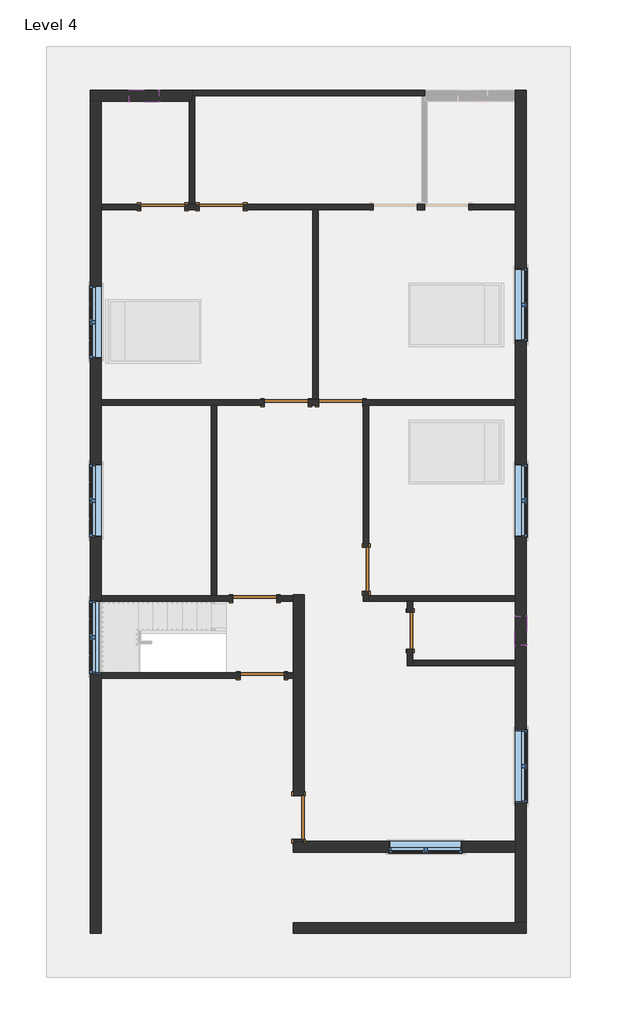
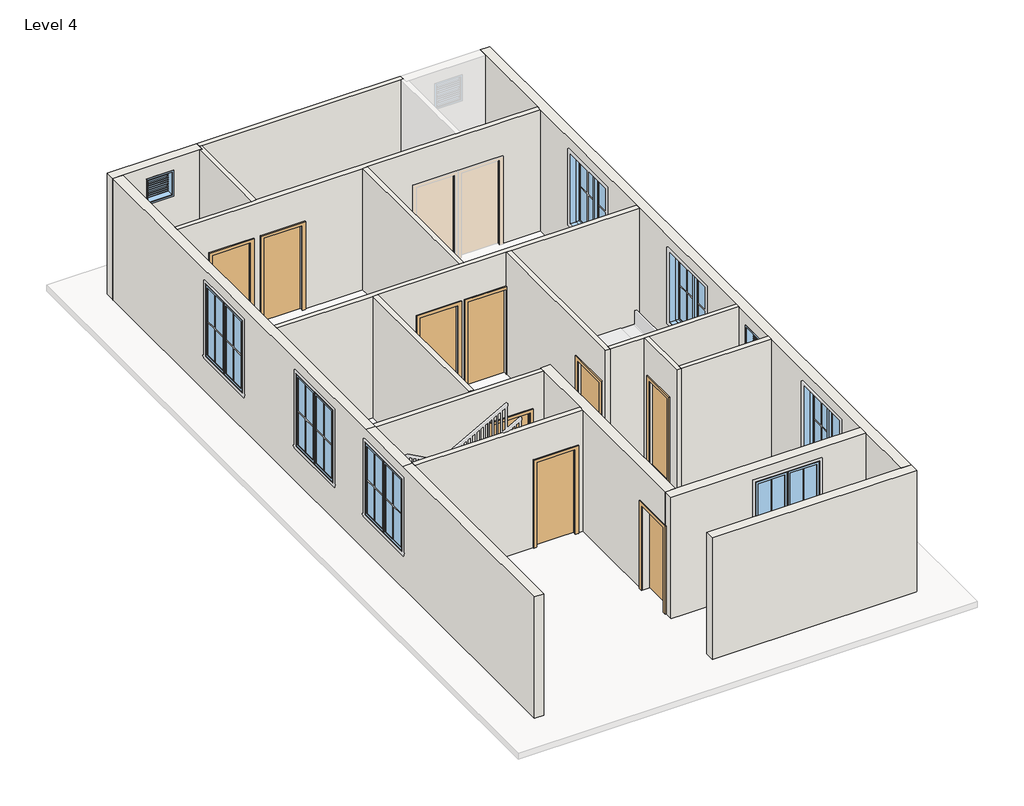
# One storey, part 1 of 3: 18 walls, 9 doors, 9 windows.
"""IFC4 building model written with IfcOpenShell, lengths in millimetres."""

from ifc_helpers import new_model, si_unit, frame, origin, place, context, project, spatial, polyline, outline, extrude, faceted_brep, transform, mapped, element, save
from components import door_78caadf7, single_flush_door_3_e5f9f3c4, single_flush_door_3_305aa2a5, single_flush_door_3_0ca8825f, window_casement_double_win_5_f93960c7, window_f2d8fef0

model = new_model("IFC4")

# Units and contexts
model_context = context("Model", 3, world=origin())
ifc_project = project(units=[si_unit("LENGTHUNIT", "METRE", prefix="MILLI")], contexts=[model_context])

# Site, building, storey
site = spatial("IfcSite", under=ifc_project)
building = spatial("IfcBuilding", under=site)
storey = spatial("IfcBuildingStorey", under=building, Name="Level 4", Elevation=6400.8)

# Doors
placement = place(None, origin())
door_shape = door_78caadf7(model_context)
element("IfcDoor", 1, ObjectType="Single-Flush : DOOR 2'6\"", at=placement, inside=storey, context=model_context, shape_type="MappedRepresentation", body=[
    mapped(door_shape, transform((860.2379845, -2779.6065691, 6400.8), x_axis=(0.0, 1.0, 0.0), y_axis=(-1.0, 0.0, 0.0), z_axis=(0.0, 0.0, 1.0))),
])
single_flush_door_3_shape = single_flush_door_3_e5f9f3c4(model_context)
element("IfcDoor", 2, ObjectType="Single-Flush : DOOR 3'", at=placement, inside=storey, context=model_context, shape_type="MappedRepresentation", body=[
    mapped(single_flush_door_3_shape, transform((-54.1620155, -1503.2565691, 6400.8), x_axis=(0.0, -1.0, 0.0), y_axis=(1.0, 0.0, 0.0), z_axis=(0.0, 0.0, 1.0))),
])
element("IfcDoor", 3, ObjectType="Single-Flush : DOOR 3'", at=placement, inside=storey, context=model_context, shape_type="MappedRepresentation", body=[
    mapped(single_flush_door_3_shape, transform((-1717.8620155, 1963.8434309, 6400.8), x_axis=(1.0, 0.0, 0.0), y_axis=(0.0, 1.0, 0.0), z_axis=(0.0, 0.0, 1.0))),
])
element("IfcDoor", 4, ObjectType="Single-Flush : DOOR 3'", at=placement, inside=storey, context=model_context, shape_type="MappedRepresentation", body=[
    mapped(single_flush_door_3_shape, transform((-2371.9120155, -2112.8565691, 6400.8), x_axis=(1.0, 0.0, 0.0), y_axis=(0.0, 1.0, 0.0), z_axis=(0.0, 0.0, 1.0))),
])
element("IfcDoor", 5, ObjectType="Single-Flush : DOOR 3'", at=placement, inside=storey, context=model_context, shape_type="MappedRepresentation", body=[
    mapped(single_flush_door_3_shape, transform((-2219.5120155, -3713.0565691, 6400.8), x_axis=(1.0, 0.0, 0.0), y_axis=(0.0, 1.0, 0.0), z_axis=(0.0, 0.0, 1.0))),
])
element("IfcDoor", 6, ObjectType="Single-Flush : DOOR 3'", at=placement, inside=storey, context=model_context, shape_type="MappedRepresentation", body=[
    mapped(single_flush_door_3_shape, transform((-4283.2620155, 6040.5434309, 6400.8), x_axis=(1.0, 0.0, 0.0), y_axis=(0.0, 1.0, 0.0), z_axis=(0.0, 0.0, 1.0))),
])
single_flush_door_3_2_shape = single_flush_door_3_305aa2a5(model_context)
element("IfcDoor", 7, ObjectType="Single-Flush : DOOR 3'", at=placement, inside=storey, context=model_context, shape_type="MappedRepresentation", body=[
    mapped(single_flush_door_3_2_shape, transform((-581.2120155, 1963.8434309, 6400.8), x_axis=(-1.0, 0.0, 0.0), y_axis=(0.0, -1.0, 0.0), z_axis=(0.0, 0.0, 1.0))),
])
element("IfcDoor", 8, ObjectType="Single-Flush : DOOR 3'", at=placement, inside=storey, context=model_context, shape_type="MappedRepresentation", body=[
    mapped(single_flush_door_3_2_shape, transform((-3064.0620155, 6040.5434309, 6400.8), x_axis=(-1.0, 0.0, 0.0), y_axis=(0.0, -1.0, 0.0), z_axis=(0.0, 0.0, 1.0))),
])
single_flush_door_3_3_shape = single_flush_door_3_0ca8825f(model_context)
element("IfcDoor", 9, ObjectType="Single-Flush : DOOR 3'", at=placement, inside=storey, context=model_context, shape_type="MappedRepresentation", body=[
    mapped(single_flush_door_3_3_shape, transform((-1457.5120155, -6665.8065691, 6400.8), x_axis=(0.0, -1.0, 0.0), y_axis=(1.0, 0.0, 0.0), z_axis=(0.0, 0.0, 1.0))),
])

# Walls
element("IfcWall", 10, ObjectType="WALL 4.5\"", at=placement, inside=storey, context=model_context, shape_type="Brep", body=[
    faceted_brep([(-3673.6620155, 8345.5934309, 6400.8), (-3616.5120155, 8345.5934309, 6400.8), (1107.8879845, 8345.5934309, 6400.8), (1165.0379845, 8345.5934309, 6400.8), (1165.0379845, 8345.5934309, 9448.8), (1107.8879845, 8345.5934309, 9448.8), (-3616.5120155, 8345.5934309, 9448.8), (-3673.6620155, 8345.5934309, 9448.8), (-3673.6620155, 8459.8934309, 6400.8), (-3673.6620155, 8459.8934309, 9448.8), (1165.0379845, 8459.8934309, 9448.8), (1165.0379845, 8459.8934309, 6400.8)], [[[0, 1, 2, 3, 4, 5, 6, 7]], [[8, 9, 10, 11]], [[3, 2, 1, 0, 8, 11]], [[4, 3, 11, 10]], [[0, 7, 9, 8]], [[7, 6, 5, 4, 10, 9]]]),
])
element("IfcWall", 11, ObjectType="WALL 4.5\"", at=placement, inside=storey, context=model_context, shape_type="SweptSolid", body=[
    extrude(outline(polyline([(-3730.8120155, 6097.6934309), (-3730.8120155, 8231.2934309), (-3673.6620155, 8231.2934309), (-3673.6620155, 8345.5934309), (-3616.5120155, 8345.5934309), (-3616.5120155, 6097.6934309), (-3730.8120155, 6097.6934309)])), frame((0.0, 0.0, 6400.8), z_axis=(0.0, 0.0, 1.0), x_axis=(1.0, 0.0, 0.0)), (0.0, 0.0, 1.0), 3048.0),
])
element("IfcWall", 12, ObjectType="WALL 4.5\"", at=placement, inside=storey, context=model_context, shape_type="Brep", body=[
    faceted_brep([(1165.0379845, 6097.6934309, 8534.4), (1165.0379845, 6097.6934309, 6400.8), (1107.8879845, 6097.6934309, 6400.8), (1012.6379845, 6097.6934309, 6400.8), (1012.6379845, 6097.6934309, 8534.4), (98.2379845, 6097.6934309, 8534.4), (98.2379845, 6097.6934309, 6400.8), (-2606.8620155, 6097.6934309, 6400.8), (-2606.8620155, 6097.6934309, 8534.4), (-3521.2620155, 6097.6934309, 8534.4), (-3521.2620155, 6097.6934309, 6400.8), (-3616.5120155, 6097.6934309, 6400.8), (-3730.8120155, 6097.6934309, 6400.8), (-3826.0620155, 6097.6934309, 6400.8), (-3826.0620155, 6097.6934309, 8534.4), (-4740.4620155, 6097.6934309, 8534.4), (-4740.4620155, 6097.6934309, 6400.8), (-5559.6120155, 6097.6934309, 6400.8), (-5559.6120155, 6097.6934309, 9448.8), (-3730.8120155, 6097.6934309, 9448.8), (-3616.5120155, 6097.6934309, 9448.8), (1107.8879845, 6097.6934309, 9448.8), (1222.1879845, 6097.6934309, 9448.8), (3050.9879845, 6097.6934309, 9448.8), (3050.9879845, 6097.6934309, 6400.8), (2079.4379845, 6097.6934309, 6400.8), (2079.4379845, 6097.6934309, 8534.4), (1012.6379845, 5983.3934309, 6400.8), (1165.0379845, 5983.3934309, 6400.8), (1165.0379845, 5983.3934309, 8534.4), (2079.4379845, 5983.3934309, 8534.4), (2079.4379845, 5983.3934309, 6400.8), (3050.9879845, 5983.3934309, 6400.8), (3050.9879845, 5983.3934309, 9448.8), (-1051.1120155, 5983.3934309, 9448.8), (-1165.4120155, 5983.3934309, 9448.8), (-5559.6120155, 5983.3934309, 9448.8), (-5559.6120155, 5983.3934309, 6400.8), (-4740.4620155, 5983.3934309, 6400.8), (-4740.4620155, 5983.3934309, 8534.4), (-3826.0620155, 5983.3934309, 8534.4), (-3826.0620155, 5983.3934309, 6400.8), (-3521.2620155, 5983.3934309, 6400.8), (-3521.2620155, 5983.3934309, 8534.4), (-2606.8620155, 5983.3934309, 8534.4), (-2606.8620155, 5983.3934309, 6400.8), (-1165.4120155, 5983.3934309, 6400.8), (-1051.1120155, 5983.3934309, 6400.8), (98.2379845, 5983.3934309, 6400.8), (98.2379845, 5983.3934309, 8534.4), (1012.6379845, 5983.3934309, 8534.4)], [[[0, 1, 2, 3, 4, 5, 6, 7, 8, 9, 10, 11, 12, 13, 14, 15, 16, 17, 18, 19, 20, 21, 22, 23, 24, 25, 26]], [[27, 28, 29, 30, 31, 32, 33, 34, 35, 36, 37, 38, 39, 40, 41, 42, 43, 44, 45, 46, 47, 48, 49, 50]], [[38, 37, 17, 16]], [[13, 12, 11, 10, 42, 41]], [[48, 47, 46, 45, 7, 6]], [[25, 24, 32, 31]], [[3, 2, 1, 28, 27]], [[18, 17, 37, 36]], [[24, 23, 33, 32]], [[14, 13, 41, 40]], [[15, 14, 40, 39]], [[16, 15, 39, 38]], [[43, 42, 10, 9]], [[44, 43, 9, 8]], [[45, 44, 8, 7]], [[4, 3, 27, 50]], [[5, 4, 50, 49]], [[6, 5, 49, 48]], [[29, 28, 1, 0]], [[30, 29, 0, 26]], [[31, 30, 26, 25]], [[23, 22, 21, 20, 19, 18, 36, 35, 34, 33]]]),
])
element("IfcWall", 13, ObjectType="WALL 4.5\"", at=placement, inside=storey, context=model_context, shape_type="SweptSolid", body=[
    extrude(outline(polyline([(-1165.4120155, 2020.9934309), (-1165.4120155, 5983.3934309), (-1051.1120155, 5983.3934309), (-1051.1120155, 2020.9934309), (-1165.4120155, 2020.9934309)])), frame((0.0, 0.0, 6400.8), z_axis=(0.0, 0.0, 1.0), x_axis=(1.0, 0.0, 0.0)), (0.0, 0.0, 1.0), 3048.0),
])
element("IfcWall", 14, ObjectType="WALL 4.5\"", at=placement, inside=storey, context=model_context, shape_type="Brep", body=[
    faceted_brep([(-1260.6620155, 1906.6934309, 8534.4), (-1260.6620155, 1906.6934309, 6400.8), (-1038.4120155, 1906.6934309, 6400.8), (-1038.4120155, 1906.6934309, 8534.4), (-124.0120155, 1906.6934309, 8534.4), (-124.0120155, 1906.6934309, 6400.8), (-111.3120155, 1906.6934309, 6400.8), (2.9879845, 1906.6934309, 6400.8), (3050.9879845, 1906.6934309, 6400.8), (3050.9879845, 1906.6934309, 9448.8), (2.9879845, 1906.6934309, 9448.8), (-111.3120155, 1906.6934309, 9448.8), (-3159.3120155, 1906.6934309, 9448.8), (-3273.6120155, 1906.6934309, 9448.8), (-5559.6120155, 1906.6934309, 9448.8), (-5559.6120155, 1906.6934309, 6400.8), (-3273.6120155, 1906.6934309, 6400.8), (-3159.3120155, 1906.6934309, 6400.8), (-2175.0620155, 1906.6934309, 6400.8), (-2175.0620155, 1906.6934309, 8534.4), (-1038.4120155, 2020.9934309, 6400.8), (-1051.1120155, 2020.9934309, 6400.8), (-1165.4120155, 2020.9934309, 6400.8), (-1260.6620155, 2020.9934309, 6400.8), (-1260.6620155, 2020.9934309, 8534.4), (-2175.0620155, 2020.9934309, 8534.4), (-2175.0620155, 2020.9934309, 6400.8), (-5559.6120155, 2020.9934309, 6400.8), (-5559.6120155, 2020.9934309, 9448.8), (-1165.4120155, 2020.9934309, 9448.8), (-1051.1120155, 2020.9934309, 9448.8), (3050.9879845, 2020.9934309, 9448.8), (3050.9879845, 2020.9934309, 6400.8), (-124.0120155, 2020.9934309, 6400.8), (-124.0120155, 2020.9934309, 8534.4), (-1038.4120155, 2020.9934309, 8534.4)], [[[0, 1, 2, 3, 4, 5, 6, 7, 8, 9, 10, 11, 12, 13, 14, 15, 16, 17, 18, 19]], [[20, 21, 22, 23, 24, 25, 26, 27, 28, 29, 30, 31, 32, 33, 34, 35]], [[33, 32, 8, 7, 6, 5]], [[2, 1, 23, 22, 21, 20]], [[18, 17, 16, 15, 27, 26]], [[15, 14, 28, 27]], [[9, 8, 32, 31]], [[3, 2, 20, 35]], [[4, 3, 35, 34]], [[5, 4, 34, 33]], [[24, 23, 1, 0]], [[25, 24, 0, 19]], [[26, 25, 19, 18]], [[14, 13, 12, 11, 10, 9, 31, 30, 29, 28]]]),
])
element("IfcWall", 15, ObjectType="WALL 4.5\"", at=placement, inside=storey, context=model_context, shape_type="SweptSolid", body=[
    extrude(outline(polyline([(-3273.6120155, -2032.8465691), (-3273.6120155, 1906.6934309), (-3159.3120155, 1906.6934309), (-3159.3120155, -2032.8465691), (-3273.6120155, -2032.8465691)])), frame((0.0, 0.0, 6400.8), z_axis=(0.0, 0.0, 1.0), x_axis=(1.0, 0.0, 0.0)), (0.0, 0.0, 1.0), 3048.0),
])
element("IfcWall", 16, ObjectType="WALL 4.5\"", at=placement, inside=storey, context=model_context, shape_type="SweptSolid", body=[
    extrude(outline(polyline([(8534.4, -1914.7120155), (6400.8, -1914.7120155), (6400.8, -1571.8120155), (9448.8, -1571.8120155), (9448.8, -5559.6120155), (6400.8, -5559.6120155), (6400.8, -2829.1120155), (8534.4, -2829.1120155), (8534.4, -1914.7120155)])), frame((0.0, -2170.0065691, 0.0), z_axis=(0.0, 1.0, 0.0), x_axis=(0.0, 0.0, 1.0)), (0.0, 0.0, 1.0), 114.3),
])
element("IfcWall", 17, ObjectType="WALL 4.5\"", at=placement, inside=storey, context=model_context, shape_type="SweptSolid", body=[
    extrude(outline(polyline([(8534.4, -1762.3120155), (6400.8, -1762.3120155), (6400.8, -1571.8120155), (9448.8, -1571.8120155), (9448.8, -5559.6120155), (6400.8, -5559.6120155), (6400.8, -2676.7120155), (8534.4, -2676.7120155), (8534.4, -1762.3120155)])), frame((0.0, -3770.2065691, 0.0), z_axis=(0.0, 1.0, 0.0), x_axis=(0.0, 0.0, 1.0)), (0.0, 0.0, 1.0), 114.3),
])
element("IfcWall", 18, ObjectType="WALL 4.5\"", at=placement, inside=storey, context=model_context, shape_type="Brep", body=[
    faceted_brep([(-111.3120155, -1960.4565691, 8534.4), (-111.3120155, -1960.4565691, 6400.8), (-111.3120155, -2170.0065691, 6400.8), (-111.3120155, -2170.0065691, 9448.8), (-111.3120155, 1906.6934309, 9448.8), (-111.3120155, 1906.6934309, 6400.8), (-111.3120155, -1046.0565691, 6400.8), (-111.3120155, -1046.0565691, 8534.4), (2.9879845, -2170.0065691, 6400.8), (2.9879845, -2055.7065691, 6400.8), (2.9879845, -1960.4565691, 6400.8), (2.9879845, -1960.4565691, 8534.4), (2.9879845, -1046.0565691, 8534.4), (2.9879845, -1046.0565691, 6400.8), (2.9879845, 1906.6934309, 6400.8), (2.9879845, 1906.6934309, 9448.8), (2.9879845, -2055.7065691, 9448.8), (2.9879845, -2170.0065691, 9448.8)], [[[0, 1, 2, 3, 4, 5, 6, 7]], [[8, 9, 10, 11, 12, 13, 14, 15, 16, 17]], [[6, 5, 14, 13]], [[2, 1, 10, 9, 8]], [[5, 4, 15, 14]], [[3, 2, 8, 17]], [[11, 10, 1, 0]], [[12, 11, 0, 7]], [[13, 12, 7, 6]], [[4, 3, 17, 16, 15]]]),
])
element("IfcWall", 19, ObjectType="WALL 4.5\"", at=placement, inside=storey, context=model_context, shape_type="Brep", body=[
    faceted_brep([(2.9879845, -2170.0065691, 6400.8), (803.0879845, -2170.0065691, 6400.8), (917.3879845, -2170.0065691, 6400.8), (3050.9879845, -2170.0065691, 6400.8), (3050.9879845, -2170.0065691, 9448.8), (917.3879845, -2170.0065691, 9448.8), (803.0879845, -2170.0065691, 9448.8), (2.9879845, -2170.0065691, 9448.8), (2.9879845, -2055.7065691, 6400.8), (2.9879845, -2055.7065691, 9448.8), (3050.9879845, -2055.7065691, 9448.8), (3050.9879845, -2055.7065691, 6400.8)], [[[0, 1, 2, 3, 4, 5, 6, 7]], [[8, 9, 10, 11]], [[3, 2, 1, 0, 8, 11]], [[0, 7, 9, 8]], [[4, 3, 11, 10]], [[7, 6, 5, 4, 10, 9]]]),
])
element("IfcWall", 20, ObjectType="WALL 4.5\"", at=placement, inside=storey, context=model_context, shape_type="Brep", body=[
    faceted_brep([(803.0879845, -2170.0065691, 6400.8), (803.0879845, -2398.6065691, 6400.8), (803.0879845, -2398.6065691, 8534.4), (803.0879845, -3160.6065691, 8534.4), (803.0879845, -3160.6065691, 6400.8), (803.0879845, -3503.5065691, 6400.8), (803.0879845, -3503.5065691, 9448.8), (803.0879845, -2170.0065691, 9448.8), (917.3879845, -2398.6065691, 8534.4), (917.3879845, -2398.6065691, 6400.8), (917.3879845, -2170.0065691, 6400.8), (917.3879845, -2170.0065691, 9448.8), (917.3879845, -3389.2065691, 9448.8), (917.3879845, -3503.5065691, 9448.8), (917.3879845, -3503.5065691, 6400.8), (917.3879845, -3389.2065691, 6400.8), (917.3879845, -3160.6065691, 6400.8), (917.3879845, -3160.6065691, 8534.4)], [[[0, 1, 2, 3, 4, 5, 6, 7]], [[8, 9, 10, 11, 12, 13, 14, 15, 16, 17]], [[10, 9, 1, 0]], [[16, 15, 14, 5, 4]], [[0, 7, 11, 10]], [[6, 5, 14, 13]], [[2, 1, 9, 8]], [[3, 2, 8, 17]], [[4, 3, 17, 16]], [[7, 6, 13, 12, 11]]]),
])
element("IfcWall", 21, ObjectType="WALL 4.5\"", at=placement, inside=storey, context=model_context, shape_type="SweptSolid", body=[
    extrude(outline(polyline([(917.3879845, -3389.2065691), (3050.9879845, -3389.2065691), (3050.9879845, -3503.5065691), (917.3879845, -3503.5065691), (917.3879845, -3389.2065691)])), frame((0.0, 0.0, 6400.8), z_axis=(0.0, 0.0, 1.0), x_axis=(1.0, 0.0, 0.0)), (0.0, 0.0, 1.0), 3048.0),
])
element("IfcWall", 22, ObjectType="WALL 9\"", at=placement, inside=storey, context=model_context, shape_type="Brep", body=[
    faceted_brep([(-3673.6620155, 8459.8934309, 6400.8), (-5788.2120155, 8459.8934309, 6400.8), (-5788.2120155, 8459.8934309, 9448.8), (-3673.6620155, 8459.8934309, 9448.8), (-4978.5870155, 8459.8934309, 9144.0), (-4978.5870155, 8459.8934309, 8534.4), (-4368.9870155, 8459.8934309, 8534.4), (-4368.9870155, 8459.8934309, 9144.0), (-3673.6620155, 8231.2934309, 6400.8), (-3673.6620155, 8231.2934309, 9448.8), (-3730.8120155, 8231.2934309, 9448.8), (-5559.6120155, 8231.2934309, 9448.8), (-5788.2120155, 8231.2934309, 9448.8), (-5788.2120155, 8231.2934309, 6400.8), (-5559.6120155, 8231.2934309, 6400.8), (-3730.8120155, 8231.2934309, 6400.8), (-4978.5870155, 8231.2934309, 9144.0), (-4368.9870155, 8231.2934309, 9144.0), (-4368.9870155, 8231.2934309, 8534.4), (-4978.5870155, 8231.2934309, 8534.4), (-3673.6620155, 8345.5934309, 6400.8), (-3673.6620155, 8345.5934309, 9448.8)], [[[0, 1, 2, 3], [4, 5, 6, 7]], [[8, 9, 10, 11, 12, 13, 14, 15], [16, 17, 18, 19]], [[1, 0, 20, 8, 15, 14, 13]], [[0, 3, 21, 9, 8, 20]], [[2, 1, 13, 12]], [[5, 4, 16, 19]], [[6, 5, 19, 18]], [[7, 6, 18, 17]], [[4, 7, 17, 16]], [[3, 2, 12, 11, 10, 9, 21]]]),
])
element("IfcWall", 23, ObjectType="WALL 9\"", at=placement, inside=storey, context=model_context, shape_type="Brep", body=[
    faceted_brep([(-5788.2120155, 8231.2934309, 6400.8), (-5788.2120155, -9078.8065691, 6400.8), (-5788.2120155, -9078.8065691, 9448.8), (-5788.2120155, -3674.9565691, 9448.8), (-5788.2120155, -2150.9565691, 9448.8), (-5788.2120155, 8231.2934309, 9448.8), (-5788.2120155, 4402.2434309, 9144.0), (-5788.2120155, 2878.2434309, 9144.0), (-5788.2120155, 2878.2434309, 7315.2), (-5788.2120155, 4402.2434309, 7315.2), (-5788.2120155, -2150.9565691, 9144.0), (-5788.2120155, -3674.9565691, 9144.0), (-5788.2120155, -3674.9565691, 7315.2), (-5788.2120155, -2150.9565691, 7315.2), (-5788.2120155, 687.4934309, 9144.0), (-5788.2120155, -836.5065691, 9144.0), (-5788.2120155, -836.5065691, 7315.2), (-5788.2120155, 687.4934309, 7315.2), (-5559.6120155, 8231.2934309, 6400.8), (-5559.6120155, 8231.2934309, 9448.8), (-5559.6120155, 6097.6934309, 9448.8), (-5559.6120155, 5983.3934309, 9448.8), (-5559.6120155, 2020.9934309, 9448.8), (-5559.6120155, 1906.6934309, 9448.8), (-5559.6120155, -2055.7065691, 9448.8), (-5559.6120155, -2150.9565691, 9448.8), (-5559.6120155, -2170.0065691, 9448.8), (-5559.6120155, -3655.9065691, 9448.8), (-5559.6120155, -3674.9565691, 9448.8), (-5559.6120155, -3770.2065691, 9448.8), (-5559.6120155, -9078.8065691, 9448.8), (-5559.6120155, -9078.8065691, 6400.8), (-5559.6120155, -3770.2065691, 6400.8), (-5559.6120155, -3655.9065691, 6400.8), (-5559.6120155, -2170.0065691, 6400.8), (-5559.6120155, -2055.7065691, 6400.8), (-5559.6120155, 1906.6934309, 6400.8), (-5559.6120155, 2020.9934309, 6400.8), (-5559.6120155, 5983.3934309, 6400.8), (-5559.6120155, 6097.6934309, 6400.8), (-5559.6120155, 4402.2434309, 9144.0), (-5559.6120155, 4402.2434309, 7315.2), (-5559.6120155, 2878.2434309, 7315.2), (-5559.6120155, 2878.2434309, 9144.0), (-5559.6120155, -2150.9565691, 9144.0), (-5559.6120155, -2150.9565691, 7315.2), (-5559.6120155, -3674.9565691, 7315.2), (-5559.6120155, -3674.9565691, 9144.0), (-5559.6120155, 687.4934309, 9144.0), (-5559.6120155, 687.4934309, 7315.2), (-5559.6120155, -836.5065691, 7315.2), (-5559.6120155, -836.5065691, 9144.0)], [[[0, 1, 2, 3, 4, 5], [6, 7, 8, 9], [10, 11, 12, 13], [14, 15, 16, 17]], [[18, 19, 20, 21, 22, 23, 24, 25, 26, 27, 28, 29, 30, 31, 32, 33, 34, 35, 36, 37, 38, 39], [40, 41, 42, 43], [44, 45, 46, 47], [48, 49, 50, 51]], [[1, 0, 18, 39, 38, 37, 36, 35, 34, 33, 32, 31]], [[2, 1, 31, 30]], [[0, 5, 19, 18]], [[41, 40, 6, 9]], [[42, 41, 9, 8]], [[43, 42, 8, 7]], [[40, 43, 7, 6]], [[45, 44, 10, 13]], [[46, 45, 13, 12]], [[47, 46, 12, 11]], [[44, 47, 11, 10]], [[49, 48, 14, 17]], [[50, 49, 17, 16]], [[51, 50, 16, 15]], [[48, 51, 15, 14]], [[4, 3, 28, 27, 26, 25]], [[3, 2, 30, 29, 28]], [[5, 4, 25, 24, 23, 22, 21, 20, 19]]]),
])
element("IfcWall", 24, ObjectType="WALL 9\"", at=placement, inside=storey, context=model_context, shape_type="Brep", body=[
    faceted_brep([(-1571.8120155, -9078.8065691, 6400.8), (3279.5879845, -9078.8065691, 6400.8), (3279.5879845, -9078.8065691, 9448.8), (-1571.8120155, -9078.8065691, 9448.8), (-1571.8120155, -8850.2065691, 6400.8), (-1571.8120155, -8850.2065691, 9448.8), (3050.9879845, -8850.2065691, 9448.8), (3279.5879845, -8850.2065691, 9448.8), (3279.5879845, -8850.2065691, 6400.8), (3050.9879845, -8850.2065691, 6400.8)], [[[0, 1, 2, 3]], [[4, 5, 6, 7, 8, 9]], [[1, 0, 4, 9, 8]], [[0, 3, 5, 4]], [[2, 1, 8, 7]], [[3, 2, 7, 6, 5]]]),
])
element("IfcWall", 25, ObjectType="WALL 9\"", at=placement, inside=storey, context=model_context, shape_type="Brep", body=[
    faceted_brep([(3279.5879845, -8850.2065691, 6400.8), (3279.5879845, 8459.8934309, 6400.8), (3279.5879845, 8459.8934309, 9448.8), (3279.5879845, -8850.2065691, 9448.8), (3279.5879845, 3240.1934309, 9144.0), (3279.5879845, 4764.1934309, 9144.0), (3279.5879845, 4764.1934309, 7315.2), (3279.5879845, 3240.1934309, 7315.2), (3279.5879845, -836.5065691, 9144.0), (3279.5879845, 687.4934309, 9144.0), (3279.5879845, 687.4934309, 7315.2), (3279.5879845, -836.5065691, 7315.2), (3279.5879845, -6361.0065691, 9144.0), (3279.5879845, -4837.0065691, 9144.0), (3279.5879845, -4837.0065691, 7315.2), (3279.5879845, -6361.0065691, 7315.2), (3279.5879845, -2474.8065691, 9144.0), (3279.5879845, -2474.8065691, 8534.4), (3279.5879845, -3084.4065691, 8534.4), (3279.5879845, -3084.4065691, 9144.0), (3050.9879845, -8850.2065691, 6400.8), (3050.9879845, -8850.2065691, 9448.8), (3050.9879845, -7389.7065691, 9448.8), (3050.9879845, -7161.1065691, 9448.8), (3050.9879845, -3503.5065691, 9448.8), (3050.9879845, -3389.2065691, 9448.8), (3050.9879845, -2170.0065691, 9448.8), (3050.9879845, -2055.7065691, 9448.8), (3050.9879845, 1906.6934309, 9448.8), (3050.9879845, 2020.9934309, 9448.8), (3050.9879845, 5983.3934309, 9448.8), (3050.9879845, 6097.6934309, 9448.8), (3050.9879845, 8231.2934309, 9448.8), (3050.9879845, 8459.8934309, 9448.8), (3050.9879845, 8459.8934309, 6400.8), (3050.9879845, 8231.2934309, 6400.8), (3050.9879845, 6097.6934309, 6400.8), (3050.9879845, 5983.3934309, 6400.8), (3050.9879845, 2020.9934309, 6400.8), (3050.9879845, 1906.6934309, 6400.8), (3050.9879845, -2055.7065691, 6400.8), (3050.9879845, -2170.0065691, 6400.8), (3050.9879845, -3389.2065691, 6400.8), (3050.9879845, -3503.5065691, 6400.8), (3050.9879845, -7161.1065691, 6400.8), (3050.9879845, -7389.7065691, 6400.8), (3050.9879845, 3240.1934309, 9144.0), (3050.9879845, 3240.1934309, 7315.2), (3050.9879845, 4764.1934309, 7315.2), (3050.9879845, 4764.1934309, 9144.0), (3050.9879845, -836.5065691, 9144.0), (3050.9879845, -836.5065691, 7315.2), (3050.9879845, 687.4934309, 7315.2), (3050.9879845, 687.4934309, 9144.0), (3050.9879845, -6361.0065691, 9144.0), (3050.9879845, -6361.0065691, 7315.2), (3050.9879845, -4837.0065691, 7315.2), (3050.9879845, -4837.0065691, 9144.0), (3050.9879845, -2474.8065691, 9144.0), (3050.9879845, -3084.4065691, 9144.0), (3050.9879845, -3084.4065691, 8534.4), (3050.9879845, -2474.8065691, 8534.4)], [[[0, 1, 2, 3], [4, 5, 6, 7], [8, 9, 10, 11], [12, 13, 14, 15], [16, 17, 18, 19]], [[20, 21, 22, 23, 24, 25, 26, 27, 28, 29, 30, 31, 32, 33, 34, 35, 36, 37, 38, 39, 40, 41, 42, 43, 44, 45], [46, 47, 48, 49], [50, 51, 52, 53], [54, 55, 56, 57], [58, 59, 60, 61]], [[1, 0, 20, 45, 44, 43, 42, 41, 40, 39, 38, 37, 36, 35, 34]], [[0, 3, 21, 20]], [[2, 1, 34, 33]], [[47, 46, 4, 7]], [[48, 47, 7, 6]], [[49, 48, 6, 5]], [[46, 49, 5, 4]], [[51, 50, 8, 11]], [[52, 51, 11, 10]], [[53, 52, 10, 9]], [[50, 53, 9, 8]], [[55, 54, 12, 15]], [[56, 55, 15, 14]], [[57, 56, 14, 13]], [[54, 57, 13, 12]], [[17, 16, 58, 61]], [[18, 17, 61, 60]], [[19, 18, 60, 59]], [[16, 19, 59, 58]], [[3, 2, 33, 32, 31, 30, 29, 28, 27, 26, 25, 24, 23, 22, 21]]]),
])
element("IfcWall", 26, ObjectType="WALL 9\"", at=placement, inside=storey, context=model_context, shape_type="Brep", body=[
    faceted_brep([(3050.9879845, -7161.1065691, 6400.8), (-1343.2120155, -7161.1065691, 6400.8), (-1571.8120155, -7161.1065691, 6400.8), (-1571.8120155, -7161.1065691, 9448.8), (-1343.2120155, -7161.1065691, 9448.8), (3050.9879845, -7161.1065691, 9448.8), (422.0879845, -7161.1065691, 9144.0), (422.0879845, -7161.1065691, 7315.2), (1946.0879845, -7161.1065691, 7315.2), (1946.0879845, -7161.1065691, 9144.0), (3050.9879845, -7389.7065691, 6400.8), (3050.9879845, -7389.7065691, 9448.8), (-1571.8120155, -7389.7065691, 9448.8), (-1571.8120155, -7389.7065691, 6400.8), (422.0879845, -7389.7065691, 9144.0), (1946.0879845, -7389.7065691, 9144.0), (1946.0879845, -7389.7065691, 7315.2), (422.0879845, -7389.7065691, 7315.2)], [[[0, 1, 2, 3, 4, 5], [6, 7, 8, 9]], [[10, 11, 12, 13], [14, 15, 16, 17]], [[2, 1, 0, 10, 13]], [[0, 5, 11, 10]], [[3, 2, 13, 12]], [[7, 6, 14, 17]], [[8, 7, 17, 16]], [[9, 8, 16, 15]], [[6, 9, 15, 14]], [[5, 4, 3, 12, 11]]]),
])
element("IfcWall", 27, ObjectType="WALL 9\"", at=placement, inside=storey, context=model_context, shape_type="Brep", body=[
    faceted_brep([(-1343.2120155, -7161.1065691, 6400.8), (-1343.2120155, -7123.0065691, 6400.8), (-1343.2120155, -7123.0065691, 8534.4), (-1343.2120155, -6208.6065691, 8534.4), (-1343.2120155, -6208.6065691, 6400.8), (-1343.2120155, -2032.8465691, 6400.8), (-1343.2120155, -2032.8465691, 9448.8), (-1343.2120155, -7161.1065691, 9448.8), (-1571.8120155, -7123.0065691, 8534.4), (-1571.8120155, -7123.0065691, 6400.8), (-1571.8120155, -7161.1065691, 6400.8), (-1571.8120155, -7161.1065691, 9448.8), (-1571.8120155, -3770.2065691, 9448.8), (-1571.8120155, -3655.9065691, 9448.8), (-1571.8120155, -2170.0065691, 9448.8), (-1571.8120155, -2055.7065691, 9448.8), (-1571.8120155, -2032.8465691, 9448.8), (-1571.8120155, -2032.8465691, 6400.8), (-1571.8120155, -2055.7065691, 6400.8), (-1571.8120155, -2170.0065691, 6400.8), (-1571.8120155, -3655.9065691, 6400.8), (-1571.8120155, -3770.2065691, 6400.8), (-1571.8120155, -6208.6065691, 6400.8), (-1571.8120155, -6208.6065691, 8534.4)], [[[0, 1, 2, 3, 4, 5, 6, 7]], [[8, 9, 10, 11, 12, 13, 14, 15, 16, 17, 18, 19, 20, 21, 22, 23]], [[10, 9, 1, 0]], [[22, 21, 20, 19, 18, 17, 5, 4]], [[6, 5, 17, 16]], [[0, 7, 11, 10]], [[2, 1, 9, 8]], [[3, 2, 8, 23]], [[4, 3, 23, 22]], [[7, 6, 16, 15, 14, 13, 12, 11]]]),
])

# Windows
window_casement_double_win_5_shape = window_casement_double_win_5_f93960c7(model_context)
element("IfcWindow", 28, ObjectType="Window-Casement-Double : WIN 5'", at=placement, inside=storey, context=model_context, shape_type="MappedRepresentation", body=[
    mapped(window_casement_double_win_5_shape, transform((-5673.9120155, 3640.2434309, 6400.8), x_axis=(0.0, 1.0, 0.0), y_axis=(-1.0, 0.0, 0.0), z_axis=(0.0, 0.0, 1.0))),
])
element("IfcWindow", 29, ObjectType="Window-Casement-Double : WIN 5'", at=placement, inside=storey, context=model_context, shape_type="MappedRepresentation", body=[
    mapped(window_casement_double_win_5_shape, transform((3165.2879845, 4002.1934309, 6400.8), x_axis=(0.0, -1.0, 0.0), y_axis=(1.0, 0.0, 0.0), z_axis=(0.0, 0.0, 1.0))),
])
element("IfcWindow", 30, ObjectType="Window-Casement-Double : WIN 5'", at=placement, inside=storey, context=model_context, shape_type="MappedRepresentation", body=[
    mapped(window_casement_double_win_5_shape, transform((3165.2879845, -74.5065691, 6400.8), x_axis=(0.0, -1.0, 0.0), y_axis=(1.0, 0.0, 0.0), z_axis=(0.0, 0.0, 1.0))),
])
element("IfcWindow", 31, ObjectType="Window-Casement-Double : WIN 5'", at=placement, inside=storey, context=model_context, shape_type="MappedRepresentation", body=[
    mapped(window_casement_double_win_5_shape, transform((3165.2879845, -5599.0065691, 6400.8), x_axis=(0.0, -1.0, 0.0), y_axis=(1.0, 0.0, 0.0), z_axis=(0.0, 0.0, 1.0))),
])
element("IfcWindow", 32, ObjectType="Window-Casement-Double : WIN 5'", at=placement, inside=storey, context=model_context, shape_type="MappedRepresentation", body=[
    mapped(window_casement_double_win_5_shape, transform((1184.0879845, -7275.4065691, 6400.8), x_axis=(-1.0, 0.0, 0.0), y_axis=(0.0, -1.0, 0.0), z_axis=(0.0, 0.0, 1.0))),
])
element("IfcWindow", 33, ObjectType="Window-Casement-Double : WIN 5'", at=placement, inside=storey, context=model_context, shape_type="MappedRepresentation", body=[
    mapped(window_casement_double_win_5_shape, transform((-5673.9120155, -2912.9565691, 6400.8), x_axis=(0.0, 1.0, 0.0), y_axis=(-1.0, 0.0, 0.0), z_axis=(0.0, 0.0, 1.0))),
])
element("IfcWindow", 34, ObjectType="Window-Casement-Double : WIN 5'", at=placement, inside=storey, context=model_context, shape_type="MappedRepresentation", body=[
    mapped(window_casement_double_win_5_shape, transform((-5673.9120155, -74.5065691, 6400.8), x_axis=(0.0, 1.0, 0.0), y_axis=(-1.0, 0.0, 0.0), z_axis=(0.0, 0.0, 1.0))),
])
window_shape = window_f2d8fef0(model_context)
element("IfcWindow", 35, ObjectType="Window-Louvers : 24\" x 24\"", at=placement, inside=storey, context=model_context, shape_type="MappedRepresentation", body=[
    mapped(window_shape, transform((-4673.7870155, 8351.9434309, 7620.0), x_axis=(1.0, 0.0, 0.0), y_axis=(0.0, 1.0, 0.0), z_axis=(0.0, 0.0, 1.0))),
])
element("IfcWindow", 36, ObjectType="Window-Louvers : 24\" x 24\"", at=placement, inside=storey, context=model_context, shape_type="MappedRepresentation", body=[
    mapped(window_shape, transform((3171.6379845, -2779.6065691, 7620.0), x_axis=(0.0, -1.0, 0.0), y_axis=(1.0, 0.0, 0.0), z_axis=(0.0, 0.0, 1.0))),
])

save(model, "model.ifc")

# Revit data of these elements
# Type "Single-Flush : DOOR 2'6\""
#   Type Mark = "10"
#   Construction Type Id = "MDOOR"
#   Assembly Code = "C1020"
#   Analytic Construction = "Metal"
#   Thickness = 0' - 2"
#   Heat Transfer Coefficient (U) = 0.651978 BTU/(h·ft²·°F)
#   Height = 7' - 0"
#   Trim Projection Ext = 0' - 1"
#   Trim Projection Int = 0' - 1"
#   Trim Width = 0' - 3"
#   Width = 2' - 6"
#   Define Thermal Properties by = 1
#   Door Material = Door - Panel
#   Frame Material = Door - Frame
#   Visual Light Transmittance = 0
#   Solar Heat Gain Coefficient = 0
#   Function = (empty or 0)
#   Wall Closure = (empty or 0)
# Type "Single-Flush : DOOR 3'"
#   Type Mark = "9"
#   Construction Type Id = "MDOOR"
#   Assembly Code = "C1020"
#   Analytic Construction = "Metal"
#   Thickness = 0' - 2"
#   Heat Transfer Coefficient (U) = 0.651978 BTU/(h·ft²·°F)
#   Height = 7' - 0"
#   Trim Projection Ext = 0' - 1"
#   Trim Projection Int = 0' - 1"
#   Trim Width = 0' - 3"
#   Width = 3' - 0"
#   Define Thermal Properties by = 1
#   Door Material = Door - Panel
#   Frame Material = Door - Frame
#   Visual Light Transmittance = 0
#   Solar Heat Gain Coefficient = 0
#   Function = (empty or 0)
#   Wall Closure = (empty or 0)
# Type "WALL 4.5\""
#   Assembly Code = "B2010"
#   Layers, outside or top first: 0' - 4 1/2" no material (function 1)
# Type "WALL 9\""
#   Assembly Code = "B2010"
#   Layers, outside or top first: 0' - 9" no material (function 1)
# Type "Window-Casement-Double : WIN 5'"
#   Type Mark = "18"
#   Fire Rating = "0.5h"
#   Assembly Code = "B2020100"
#   Analytic Construction = "Double glazing - domestic"
#   Frame Extension [instance default] = 0' - 0 1/4"
#   Window Inset [instance default] = 0' - 0"
#   Wall Thickness [instance default] = 0' - 6"
#   Interior Wall Closure [instance default] = 0' - 2 1/4"
#   Half Width = 2' - 6"
#   Visual Light Transmittance = 0.81
#   Thermal Resistance (R) = 1.8146 (h·ft²·°F)/BTU
#   Solar Heat Gain Coefficient = 0.76
#   Rough Width = 5' - 0 1/2"
#   Rough Height = 6' - 0 1/2"
#   Height = 6' - 0"
#   Heat Transfer Coefficient (U) = 0.5511 BTU/(h·ft²·°F)
#   Exterior Wall Closure [instance default] = 0' - 1 1/4"
#   Extension Jamb [instance default] = 0' - 2 1/4"
#   Default Sill Height = 3' - 0"
#   Width = 5' - 0"
#   Muntin Visibility = yes
#   Interior Trim Visibility [instance default] = yes
#   Exterior Trim Visibility [instance default] = yes
#   Extension Jamb Visibility [instance default] = yes
#   Interior Trim Material = Wood - Stained
#   Muntin Pattern = Muntin Pattern_2x2 : Muntin Pattern_2x2
#   Interior Trim = Trim-Window-Interior-Flat : Picture Frame
#   Interior Frame Material = Wood - Stained
#   Glass Panel Material = Glass
#   Exterior Trim Material = Clad - White
#   Exterior Trim = Trim-Window-Exterior-Flat : with Sill
#   Exterior Frame Material = Clad - White
#   Wall Closure = (empty or 0)
# Type "Window-Louvers : 24\" x 24\""
#   Type Mark = "19"
#   Construction Type Id = "GSP4R"
#   Assembly Code = "B20"
#   Analytic Construction = "1/8 in Pilkington single glazing"
#   Visual Light Transmittance = 0.9
#   Thermal Resistance (R) = 1.53941 (h·ft²·°F)/BTU
#   Solar Heat Gain Coefficient = 0.78
#   Max Height = 1' - 11.74264"
#   Height = 2' - 0"
#   Heat Transfer Coefficient (U) = 0.6496 BTU/(h·ft²·°F)
#   Blade Width [instance default] = 1' - 10 1/2"
#   Blade Vertical Thickness = 0' - 0.35355"
#   Blade Thickness = 0' - 0 1/4"
#   Blade Spacing = 0' - 1 1/2"
#   Blade Height = 0' - 1.85355"
#   Blade Depth = 0' - 3"
#   Blade Angle = 45.00°
#   Default Sill Height = 3' - 0"
#   Trim Projection_Exterior = 0' - 0 1/2"
#   Trim Projection_Interior = 0' - 0 1/2"
#   Trim Width_Exterior = 0' - 1 1/2"
#   Trim Width_Interior = 0' - 1 1/2"
#   Width = 2' - 0"
#   Max Blade Count = 12
#   Define Thermal Properties by = 1
#   Blade Count = 12
#   Frame Material = Birch
#   Louver Material = Birch
#   Trim Exterior Material = Birch
#   Trim Interior Material = Birch
#   Wall Closure = (empty or 0)
# Element 1 (IfcDoor, "Single-Flush : DOOR 2'6\"")
#   Phase Created = New Construction
#   Materials on its faces: "Door - Frame", "Door - Panel"
# Elements 2, 3, 4, 5, 6, 7, 8, 9 (IfcDoor, "Single-Flush : DOOR 3'")
#   Phase Created = New Construction
#   Materials on its faces: "Door - Frame", "Door - Panel"
# Elements 10, 17 (IfcWall, "WALL 4.5\"")
#   Top Offset = 0' - 0"
#   Base Offset = 0' - 0"
#   Unconnected Height = 10' - 0"
#   wall height = 10' - 0"
#   Phase Created = New Construction
#   Base Constraint = Level 4
#   Materials on its faces: "Default Wall", "Brick, Common"
# Elements 11, 12, 13, 14, 15, 16, 18, 19, 20, 21 (IfcWall, "WALL 4.5\"")
#   Top Offset = 0' - 0"
#   Base Offset = 0' - 0"
#   Unconnected Height = 10' - 0"
#   wall height = 10' - 0"
#   Phase Created = New Construction
#   Base Constraint = Level 4
#   Materials on its faces: "Default Wall"
# Elements 22, 23, 24, 25, 26, 27 (IfcWall, "WALL 9\"")
#   Top Offset = 0' - 0"
#   Base Offset = 0' - 0"
#   Unconnected Height = 10' - 0"
#   wall height = 10' - 0"
#   Phase Created = New Construction
#   Base Constraint = Level 4
#   Materials on its faces: "Default Wall", "Brick, Common"
# Element 28 (IfcWindow, "Window-Casement-Double : WIN 5'")
#   Mark = "21"
#   Window Inset = 0' - 0"
#   Interior Wall Closure = 0' - 2 1/4"
#   Frame Extension = 0' - 0 1/4"
#   Exterior Wall Closure = 0' - 1 1/4"
#   Interior Trim Visibility = yes
#   Exterior Trim Visibility = yes
#   Phase Created = New Construction
#   Materials on its faces: "Wood - Stained", "Glass", "Clad - White"
# Element 29 (IfcWindow, "Window-Casement-Double : WIN 5'")
#   Mark = "22"
#   Window Inset = 0' - 0"
#   Interior Wall Closure = 0' - 2 1/4"
#   Frame Extension = 0' - 0 1/4"
#   Exterior Wall Closure = 0' - 1 1/4"
#   Interior Trim Visibility = yes
#   Exterior Trim Visibility = yes
#   Phase Created = New Construction
#   Materials on its faces: "Wood - Stained", "Glass", "Clad - White"
# Element 30 (IfcWindow, "Window-Casement-Double : WIN 5'")
#   Mark = "23"
#   Window Inset = 0' - 0"
#   Interior Wall Closure = 0' - 2 1/4"
#   Frame Extension = 0' - 0 1/4"
#   Exterior Wall Closure = 0' - 1 1/4"
#   Interior Trim Visibility = yes
#   Exterior Trim Visibility = yes
#   Phase Created = New Construction
#   Materials on its faces: "Wood - Stained", "Glass", "Clad - White"
# Element 31 (IfcWindow, "Window-Casement-Double : WIN 5'")
#   Mark = "24"
#   Window Inset = 0' - 0"
#   Interior Wall Closure = 0' - 2 1/4"
#   Frame Extension = 0' - 0 1/4"
#   Exterior Wall Closure = 0' - 1 1/4"
#   Interior Trim Visibility = yes
#   Exterior Trim Visibility = yes
#   Phase Created = New Construction
#   Materials on its faces: "Wood - Stained", "Glass", "Clad - White"
# Element 32 (IfcWindow, "Window-Casement-Double : WIN 5'")
#   Mark = "25"
#   Window Inset = 0' - 0"
#   Interior Wall Closure = 0' - 2 1/4"
#   Frame Extension = 0' - 0 1/4"
#   Exterior Wall Closure = 0' - 1 1/4"
#   Interior Trim Visibility = yes
#   Exterior Trim Visibility = yes
#   Phase Created = New Construction
#   Materials on its faces: "Wood - Stained", "Glass", "Clad - White"
# Element 33 (IfcWindow, "Window-Casement-Double : WIN 5'")
#   Mark = "26"
#   Window Inset = 0' - 0"
#   Interior Wall Closure = 0' - 2 1/4"
#   Frame Extension = 0' - 0 1/4"
#   Exterior Wall Closure = 0' - 1 1/4"
#   Interior Trim Visibility = yes
#   Exterior Trim Visibility = yes
#   Phase Created = New Construction
#   Materials on its faces: "Wood - Stained", "Glass", "Clad - White"
# Element 34 (IfcWindow, "Window-Casement-Double : WIN 5'")
#   Mark = "27"
#   Window Inset = 0' - 0"
#   Interior Wall Closure = 0' - 2 1/4"
#   Frame Extension = 0' - 0 1/4"
#   Exterior Wall Closure = 0' - 1 1/4"
#   Interior Trim Visibility = yes
#   Exterior Trim Visibility = yes
#   Phase Created = New Construction
#   Materials on its faces: "Wood - Stained", "Glass", "Clad - White"
# Element 35 (IfcWindow, "Window-Louvers : 24\" x 24\"")
#   Mark = "28"
#   Blade Width = 1' - 10 1/2"
#   Phase Created = New Construction
#   Materials on its faces: "Birch"
# Element 36 (IfcWindow, "Window-Louvers : 24\" x 24\"")
#   Mark = "30"
#   Blade Width = 1' - 10 1/2"
#   Phase Created = New Construction
#   Materials on its faces: "Birch"
# Materials
#   "Door - Panel": class "Wood", colour RGB 210 159 95, transparency 0, Cost = 0
#   "Door - Frame": colour RGB 118 70 51, transparency 0, Cost = 0
#   "Wood - Stained": class "Wood", colour RGB 224 178 126, transparency 0, Cost = 0
#   "Glass": class "Glass", colour RGB 0 128 192, transparency 0.75, Description = "Soda Lime Glass", Cost = 0
#   "Clad - White": class "Wood", colour RGB 242 242 238, transparency 0, Cost = 0
#   "Birch": class "Wood", colour RGB 224 178 126, transparency 0, Description = "Betula Alleghaniensis", Cost = 0
#   "Default Wall": colour RGB 128 128 128, transparency 0, Cost = 0
#   "Brick, Common": class "Masonry", colour RGB 170 98 104, transparency 0, Description = "Common brick", Cost = 0
